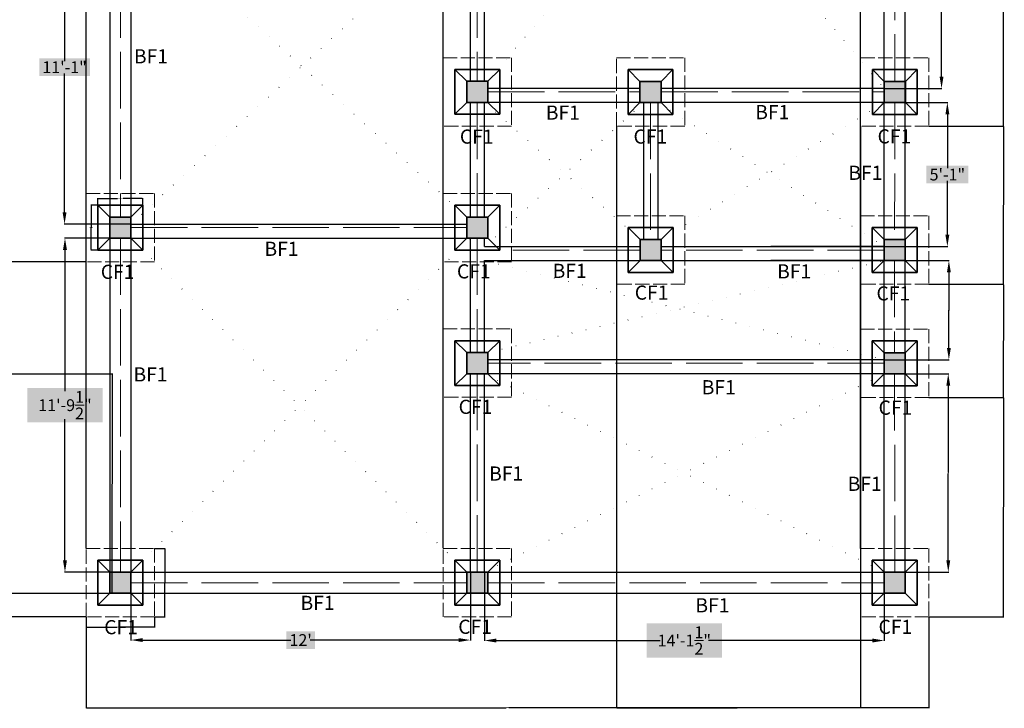
# Model space of a CAD drawing. Units: inches. Extents: x -301 to 715, y -607 to 364.
# Tile 140 of 141: x 194 to 612, y -273 to 19. Entities that reach past the tile are written whole.
import ezdxf

# ---------------------------------------------------------------- set-up
doc = ezdxf.new("R2010")
doc.units = ezdxf.units.IN
doc.header["$MEASUREMENT"] = 0
doc.linetypes.add('ACAD_ISO02W100', pattern=[15, 12, -3])
doc.linetypes.add('ACAD_ISO07W100', pattern=[3, 0, -3])
for name, color, linetype, lineweight in [('A-ANNO-DIMS', 2, 'Continuous', 18), ('S-ANNO-DIMS', 2, 'Continuous', 18), ('S-ANNO-TEXT', 240, 'Continuous', 18), ('S-BEAM-CNTR', 2, 'ACAD_ISO02W100', 13), ('S-COLS', 2, 'Continuous', 35), ('S-FNDN', 2, 'Continuous', 35), ('S-FNDN-HIDN', 220, 'ACAD_ISO02W100', 18)]:
    doc.layers.add(name, color=color, linetype=linetype, lineweight=lineweight)
for name, color, linetype, lineweight, true_color in [('S-BEAM', 152, 'Continuous', 30, 0x2776bb), ('S-COLS-PATT', 7, 'Continuous', 13, 0xffffff), ('S-FNDN-DIAG', 252, 'ACAD_ISO07W100', 13, 0x939598)]:
    doc.layers.add(name, color=color, linetype=linetype, lineweight=lineweight, true_color=true_color)
doc.styles.get("Standard").update_dxf_attribs({"font": 'arial.ttf'})
doc.dimstyles.get("Standard").update_dxf_attribs({"dimtxt": 0.18, "dimasz": 0.18, "dimexe": 0.18, "dimexo": 0.0625, "dimgap": 0.09, "dimtad": 0, "dimtih": 1, "dimtoh": 1, "dimdec": 1, "dimzin": 0, "dimdsep": 46, "dimlunit": 4, "dimtxsty": 'Standard', "dimcen": 0.09, "dimclrd": 3, "dimclre": 4, "dimclrt": 6, "dimadec": 0, "dimazin": 0, "dimtfac": 1, "dimtdec": 1, "dimtofl": 0, "dimtmove": 0, "dimatfit": 3, "dimfxl": 1, "dimtfill": 2, "dimtfillclr": 51, "dimtolj": 1, "dimtzin": 0, "dimarcsym": 0})

# ---------------------------------------------------------------- blocks, each defined once
blk = doc.blocks.new('*D58')
at = {"layer": 'Defpoints', "color": 0, "transparency": 16777216}
for p in [(391.39, -214.82), (560.9, -214.82), (560.9, -243.84)]:
    blk.add_point(p, dxfattribs=at)
at = {"layer": 'S-ANNO-DIMS', "color": 0, "lineweight": -2, "transparency": 16777216}
for p, q in [((391.39, -214.88), (391.39, -244.02)), ((560.9, -214.88), (560.9, -244.02)), ((396.39, -243.84), (465.88, -243.84)), ((555.9, -243.84), (486.41, -243.84))]:
    blk.add_line(p, q, dxfattribs=at)
at = {"layer": 'S-ANNO-DIMS', "color": 0, "transparency": 16777216}
for points in [[(396.39, -243.01), (396.39, -244.68), (391.39, -243.84)], [(555.9, -243.01), (555.9, -244.68), (560.9, -243.84)]]:
    blk.add_solid(points, dxfattribs=at)
at = {"layer": 'S-ANNO-DIMS', "color": 0, "transparency": 16777216, "insert": (476.15, -243.84), "char_height": 5, "attachment_point": 5, "bg_fill": 1, "box_fill_scale": 1.25, "bg_fill_color": 51, "bg_fill_transparency": 0}
blk.add_mtext('\\A1;14\'-1{\\H1x;\\S1/2;}"', dxfattribs=at)
blk = doc.blocks.new('*D59')
at = {"layer": 'Defpoints', "color": 0, "transparency": 16777216}
for p in [(241.39, -214.82), (385.39, -214.81), (385.39, -243.64)]:
    blk.add_point(p, dxfattribs=at)
at = {"layer": 'S-ANNO-DIMS', "color": 0, "lineweight": -2, "transparency": 16777216}
for p, q in [((241.39, -214.88), (241.39, -243.82)), ((385.39, -214.87), (385.39, -243.82)), ((246.39, -243.64), (309.29, -243.64)), ((380.39, -243.64), (317.49, -243.64))]:
    blk.add_line(p, q, dxfattribs=at)
at = {"layer": 'S-ANNO-DIMS', "color": 0, "transparency": 16777216}
for points in [[(246.39, -242.81), (246.39, -244.48), (241.39, -243.64)], [(380.39, -242.81), (380.39, -244.48), (385.39, -243.64)]]:
    blk.add_solid(points, dxfattribs=at)
at = {"layer": 'S-ANNO-DIMS', "color": 0, "transparency": 16777216, "insert": (313.39, -243.64), "char_height": 5, "attachment_point": 5, "bg_fill": 1, "box_fill_scale": 1.25, "bg_fill_color": 51, "bg_fill_transparency": 0}
blk.add_mtext("\\A1;12'", dxfattribs=at)
blk = doc.blocks.new('*D60')
at = {"layer": 'Defpoints', "color": 0, "transparency": 16777216}
for p in [(560.89, -130.82), (588.13, -130.82), (560.89, -214.82)]:
    blk.add_point(p, dxfattribs=at)
at = {"layer": 'S-ANNO-DIMS', "color": 0, "lineweight": -2, "transparency": 16777216}
for p, q in [((560.95, -130.82), (588.31, -130.82)), ((588.13, -135.82), (588.13, -172.64)), ((588.13, -209.82), (588.13, -173)), ((560.95, -214.82), (588.31, -214.82))]:
    blk.add_line(p, q, dxfattribs=at)
at = {"layer": 'S-ANNO-DIMS', "color": 0, "transparency": 16777216}
for points in [[(587.3, -135.82), (588.97, -135.82), (588.13, -130.82)], [(587.3, -209.82), (588.97, -209.82), (588.13, -214.82)]]:
    blk.add_solid(points, dxfattribs=at)
at = {"layer": 'S-ANNO-DIMS', "color": 0, "transparency": 16777216, "insert": (588.13, -172.82), "char_height": 0.18, "attachment_point": 5, "bg_fill": 1, "box_fill_scale": 1.25, "bg_fill_color": 51, "bg_fill_transparency": 0}
blk.add_mtext("\\A1;7'", dxfattribs=at)
blk = doc.blocks.new('*D61')
at = {"layer": 'Defpoints', "color": 0, "transparency": 16777216}
for p in [(560.89, -82.82), (588.39, -82.82), (560.89, -124.82)]:
    blk.add_point(p, dxfattribs=at)
at = {"layer": 'S-ANNO-DIMS', "color": 0, "lineweight": -2, "transparency": 16777216}
for p, q in [((560.95, -82.82), (588.57, -82.82)), ((588.39, -87.82), (588.39, -103.64)), ((588.39, -119.82), (588.39, -104)), ((560.95, -124.82), (588.57, -124.82))]:
    blk.add_line(p, q, dxfattribs=at)
at = {"layer": 'S-ANNO-DIMS', "color": 0, "transparency": 16777216}
for points in [[(587.56, -87.82), (589.23, -87.82), (588.39, -82.82)], [(587.56, -119.82), (589.23, -119.82), (588.39, -124.82)]]:
    blk.add_solid(points, dxfattribs=at)
at = {"layer": 'S-ANNO-DIMS', "color": 0, "transparency": 16777216, "insert": (588.39, -103.82), "char_height": 0.18, "attachment_point": 5, "bg_fill": 1, "box_fill_scale": 1.25, "bg_fill_color": 51, "bg_fill_transparency": 0}
blk.add_mtext('\\A1;3\'-6"', dxfattribs=at)
blk = doc.blocks.new('*D62')
at = {"layer": 'Defpoints', "color": 0, "transparency": 16777216}
for p in [(560.89, -15.82), (587.75, -15.82), (560.89, -76.82)]:
    blk.add_point(p, dxfattribs=at)
at = {"layer": 'S-ANNO-DIMS', "color": 0, "lineweight": -2, "transparency": 16777216}
for p, q in [((560.95, -15.82), (587.93, -15.82)), ((587.75, -20.82), (587.75, -43.67)), ((587.75, -71.82), (587.75, -48.96)), ((560.95, -76.82), (587.93, -76.82))]:
    blk.add_line(p, q, dxfattribs=at)
at = {"layer": 'S-ANNO-DIMS', "color": 0, "transparency": 16777216}
for points in [[(586.92, -20.82), (588.59, -20.82), (587.75, -15.82)], [(586.92, -71.82), (588.59, -71.82), (587.75, -76.82)]]:
    blk.add_solid(points, dxfattribs=at)
at = {"layer": 'S-ANNO-DIMS', "color": 0, "transparency": 16777216, "insert": (587.75, -46.32), "char_height": 5, "attachment_point": 5, "bg_fill": 1, "box_fill_scale": 1.25, "bg_fill_color": 51, "bg_fill_transparency": 0}
blk.add_mtext('\\A1;5\'-1"', dxfattribs=at)
blk = doc.blocks.new('*D63')
at = {"layer": 'Defpoints', "color": 0, "transparency": 16777216}
for p in [(560.89, 193.18), (585.29, 193.18), (560.89, -9.82)]:
    blk.add_point(p, dxfattribs=at)
at = {"layer": 'S-ANNO-DIMS', "color": 0, "lineweight": -2, "transparency": 16777216}
for p, q in [((560.95, 193.18), (585.47, 193.18)), ((585.29, 188.18), (585.29, 94.33)), ((585.29, -4.82), (585.29, 89.04)), ((560.95, -9.82), (585.47, -9.82))]:
    blk.add_line(p, q, dxfattribs=at)
at = {"layer": 'S-ANNO-DIMS', "color": 0, "transparency": 16777216}
for points in [[(584.46, 188.18), (586.12, 188.18), (585.29, 193.18)], [(584.46, -4.82), (586.12, -4.82), (585.29, -9.82)]]:
    blk.add_solid(points, dxfattribs=at)
at = {"layer": 'S-ANNO-DIMS', "color": 0, "transparency": 16777216, "insert": (585.29, 91.68), "char_height": 5, "attachment_point": 5, "bg_fill": 1, "box_fill_scale": 1.25, "bg_fill_color": 51, "bg_fill_transparency": 0}
blk.add_mtext('\\A1;16\'-11"', dxfattribs=at)
blk = doc.blocks.new('*D69')
at = {"layer": 'Defpoints', "color": 0, "transparency": 16777216}
for p in [(241.39, 65.68), (213.23, -67.32), (241.39, -67.32)]:
    blk.add_point(p, dxfattribs=at)
at = {"layer": 'S-ANNO-DIMS', "color": 0, "lineweight": -2, "transparency": 16777216}
for p, q in [((241.33, 65.68), (213.05, 65.68)), ((213.23, 60.68), (213.23, 1.78)), ((213.23, -62.32), (213.23, -3.42)), ((241.33, -67.32), (213.05, -67.32))]:
    blk.add_line(p, q, dxfattribs=at)
at = {"layer": 'S-ANNO-DIMS', "color": 0, "transparency": 16777216}
for points in [[(212.4, 60.68), (214.06, 60.68), (213.23, 65.68)], [(212.4, -62.32), (214.06, -62.32), (213.23, -67.32)]]:
    blk.add_solid(points, dxfattribs=at)
at = {"layer": 'S-ANNO-DIMS', "color": 0, "transparency": 16777216, "insert": (213.23, -0.82), "char_height": 5, "attachment_point": 5, "bg_fill": 1, "box_fill_scale": 1.25, "bg_fill_color": 51, "bg_fill_transparency": 0}
blk.add_mtext('\\A1;11\'-1"', dxfattribs=at)
blk = doc.blocks.new('*D70')
at = {"layer": 'Defpoints', "color": 0, "transparency": 16777216}
for p in [(241.39, -73.32), (213.4, -214.82), (241.39, -214.82)]:
    blk.add_point(p, dxfattribs=at)
at = {"layer": 'S-ANNO-DIMS', "color": 0, "lineweight": -2, "transparency": 16777216}
for p, q in [((241.33, -73.32), (213.22, -73.32)), ((213.4, -78.32), (213.4, -138.08)), ((213.4, -209.82), (213.4, -150.05)), ((241.33, -214.82), (213.22, -214.82))]:
    blk.add_line(p, q, dxfattribs=at)
at = {"layer": 'S-ANNO-DIMS', "color": 0, "transparency": 16777216}
for points in [[(212.56, -78.32), (214.23, -78.32), (213.4, -73.32)], [(212.56, -209.82), (214.23, -209.82), (213.4, -214.82)]]:
    blk.add_solid(points, dxfattribs=at)
at = {"layer": 'S-ANNO-DIMS', "color": 0, "transparency": 16777216, "insert": (213.4, -144.07), "char_height": 5, "attachment_point": 5, "bg_fill": 1, "box_fill_scale": 1.25, "bg_fill_color": 51, "bg_fill_transparency": 0}
blk.add_mtext('\\A1;11\'-9{\\H1x;\\S1/2;}"', dxfattribs=at)
blk = doc.blocks.new('CF1-BASE-29')
at = {"ltscale": 0.5}
for p, q in [((0, 0), (0, 29)), ((0, 29), (29, 29)), ((29, 29), (29, 0)), ((29, 0), (0, 0))]:
    blk.add_line(p, q, dxfattribs=at)
blk = doc.blocks.new('CF1-SLOPED-PAD')
for p, q in [((0, 0), (0, 19)), ((0, 19), (19, 19)), ((0, 19), (5, 14)), ((14, 14), (19, 19)), ((19, 19), (19, 0)), ((0, 0), (5, 5)), ((14, 5), (19, 0)), ((19, 0), (0, 0))]:
    blk.add_line(p, q)
blk = doc.blocks.new('*D92')
at = {"layer": 'A-ANNO-DIMS', "color": 4, "lineweight": -2, "transparency": 16777216}
for p, q in [((222.39, -233.88), (222.39, -238.35)), ((251.39, -233.88), (251.39, -238.35))]:
    blk.add_line(p, q, dxfattribs=at)
at = {"layer": 'A-ANNO-DIMS', "color": 3, "lineweight": -2, "transparency": 16777216}
for p, q in [((222.57, -238.17), (235.61, -238.17)), ((251.21, -238.17), (238.17, -238.17))]:
    blk.add_line(p, q, dxfattribs=at)
at = {"layer": 'A-ANNO-DIMS', "color": 3, "transparency": 16777216}
for points in [[(222.57, -238.14), (222.57, -238.2), (222.39, -238.17)], [(251.21, -238.14), (251.21, -238.2), (251.39, -238.17)]]:
    blk.add_solid(points, dxfattribs=at)
at = {"layer": 'Defpoints', "color": 0, "transparency": 16777216}
for p in [(222.39, -233.82), (251.39, -233.82), (251.39, -238.17)]:
    blk.add_point(p, dxfattribs=at)
at = {"layer": 'A-ANNO-DIMS', "color": 6, "transparency": 16777216, "insert": (236.89, -238.17), "char_height": 0.18, "attachment_point": 5, "bg_fill": 1, "box_fill_scale": 1.25, "bg_fill_color": 51, "bg_fill_transparency": 0}
blk.add_mtext('\\A1;CF1 BASE 2\'-5" TYP.', dxfattribs=at)
blk = doc.blocks.new('*D93')
at = {"layer": 'A-ANNO-DIMS', "color": 4, "lineweight": -2, "transparency": 16777216}
for p, q in [((251.45, -204.82), (255.92, -204.82)), ((251.45, -233.82), (255.92, -233.82))]:
    blk.add_line(p, q, dxfattribs=at)
at = {"layer": 'A-ANNO-DIMS', "color": 3, "lineweight": -2, "transparency": 16777216}
for p, q in [((255.74, -205), (255.74, -219.14)), ((255.74, -233.64), (255.74, -219.5))]:
    blk.add_line(p, q, dxfattribs=at)
at = {"layer": 'A-ANNO-DIMS', "color": 3, "transparency": 16777216}
for points in [[(255.71, -205), (255.77, -205), (255.74, -204.82)], [(255.71, -233.64), (255.77, -233.64), (255.74, -233.82)]]:
    blk.add_solid(points, dxfattribs=at)
at = {"layer": 'Defpoints', "color": 0, "transparency": 16777216}
for p in [(251.39, -204.82), (255.74, -204.82), (251.39, -233.82)]:
    blk.add_point(p, dxfattribs=at)
at = {"layer": 'A-ANNO-DIMS', "color": 6, "transparency": 16777216, "insert": (255.74, -219.32), "char_height": 0.18, "attachment_point": 5, "bg_fill": 1, "box_fill_scale": 1.25, "bg_fill_color": 51, "bg_fill_transparency": 0}
blk.add_mtext('\\A1;2\'-5" TYP.', dxfattribs=at)
blk = doc.blocks.new('*D94')
at = {"layer": 'A-ANNO-DIMS', "color": 4, "lineweight": -2, "transparency": 16777216}
for p, q in [((227.39, -59.26), (227.39, -56.29)), ((246.39, -59.26), (246.39, -56.29))]:
    blk.add_line(p, q, dxfattribs=at)
at = {"layer": 'A-ANNO-DIMS', "color": 3, "lineweight": -2, "transparency": 16777216}
for p, q in [((227.57, -56.47), (235.69, -56.47)), ((246.21, -56.47), (238.09, -56.47))]:
    blk.add_line(p, q, dxfattribs=at)
at = {"layer": 'A-ANNO-DIMS', "color": 3, "transparency": 16777216}
for points in [[(227.57, -56.44), (227.57, -56.5), (227.39, -56.47)], [(246.21, -56.44), (246.21, -56.5), (246.39, -56.47)]]:
    blk.add_solid(points, dxfattribs=at)
at = {"layer": 'Defpoints', "color": 0, "transparency": 16777216}
for p in [(227.39, -56.47), (227.39, -59.32), (246.39, -59.32)]:
    blk.add_point(p, dxfattribs=at)
at = {"layer": 'A-ANNO-DIMS', "color": 6, "transparency": 16777216, "insert": (236.89, -56.47), "char_height": 0.18, "attachment_point": 5, "bg_fill": 1, "box_fill_scale": 1.25, "bg_fill_color": 51, "bg_fill_transparency": 0}
blk.add_mtext('\\A1;CF1 PAD 1\'-7" TYP.', dxfattribs=at)
blk = doc.blocks.new('*D95')
at = {"layer": 'A-ANNO-DIMS', "color": 4, "lineweight": -2, "transparency": 16777216}
for p, q in [((227.33, -59.32), (224.36, -59.32)), ((227.33, -78.32), (224.36, -78.32))]:
    blk.add_line(p, q, dxfattribs=at)
at = {"layer": 'A-ANNO-DIMS', "color": 3, "lineweight": -2, "transparency": 16777216}
for p, q in [((224.54, -59.5), (224.54, -68.64)), ((224.54, -78.14), (224.54, -69))]:
    blk.add_line(p, q, dxfattribs=at)
at = {"layer": 'A-ANNO-DIMS', "color": 3, "transparency": 16777216}
for points in [[(224.51, -59.5), (224.57, -59.5), (224.54, -59.32)], [(224.51, -78.14), (224.57, -78.14), (224.54, -78.32)]]:
    blk.add_solid(points, dxfattribs=at)
at = {"layer": 'Defpoints', "color": 0, "transparency": 16777216}
for p in [(227.39, -59.32), (224.54, -78.32), (227.39, -78.32)]:
    blk.add_point(p, dxfattribs=at)
at = {"layer": 'A-ANNO-DIMS', "color": 6, "transparency": 16777216, "insert": (224.54, -68.82), "char_height": 0.18, "attachment_point": 5, "bg_fill": 1, "box_fill_scale": 1.25, "bg_fill_color": 51, "bg_fill_transparency": 0}
blk.add_mtext('\\A1;1\'-7" TYP.', dxfattribs=at)
blk = doc.blocks.new('*D152')
at = {"layer": 'A-ANNO-DIMS', "color": 4, "lineweight": -2, "transparency": 16777216}
for p, q in [((123.96, -130.82), (233.66, -130.82)), ((132.96, -223.82), (233.66, -223.82))]:
    blk.add_line(p, q, dxfattribs=at)
at = {"layer": 'A-ANNO-DIMS', "color": 3, "lineweight": -2, "transparency": 16777216}
for p, q in [((233.48, -131), (233.48, -177.14)), ((233.48, -223.64), (233.48, -177.5))]:
    blk.add_line(p, q, dxfattribs=at)
at = {"layer": 'A-ANNO-DIMS', "color": 3, "transparency": 16777216}
for points in [[(233.45, -131), (233.51, -131), (233.48, -130.82)], [(233.45, -223.64), (233.51, -223.64), (233.48, -223.82)]]:
    blk.add_solid(points, dxfattribs=at)
at = {"layer": 'Defpoints', "color": 0, "transparency": 16777216}
for p in [(123.9, -130.82), (233.48, -130.82), (132.9, -223.82)]:
    blk.add_point(p, dxfattribs=at)
at = {"layer": 'A-ANNO-DIMS', "color": 6, "transparency": 16777216, "insert": (233.48, -177.32), "char_height": 0.18, "attachment_point": 5, "bg_fill": 1, "box_fill_scale": 1.25, "bg_fill_color": 51, "bg_fill_transparency": 0}
blk.add_mtext('\\A1;7\'-9"', dxfattribs=at)
blk = doc.blocks.new('*D161')
at = {"layer": 'A-ANNO-DIMS', "color": 4, "lineweight": -2, "transparency": 16777216}
for p, q in [((222.39, -233.88), (222.39, -272.48)), ((579.9, -233.89), (579.9, -272.48))]:
    blk.add_line(p, q, dxfattribs=at)
at = {"layer": 'A-ANNO-DIMS', "color": 3, "lineweight": -2, "transparency": 16777216}
for p, q in [((222.57, -272.3), (400.54, -272.3)), ((579.72, -272.3), (401.76, -272.3))]:
    blk.add_line(p, q, dxfattribs=at)
at = {"layer": 'A-ANNO-DIMS', "color": 3, "transparency": 16777216}
for points in [[(222.57, -272.27), (222.57, -272.33), (222.39, -272.3)], [(579.72, -272.27), (579.72, -272.33), (579.9, -272.3)]]:
    blk.add_solid(points, dxfattribs=at)
at = {"layer": 'Defpoints', "color": 0, "transparency": 16777216}
for p in [(222.39, -233.82), (579.9, -233.83), (579.9, -272.3)]:
    blk.add_point(p, dxfattribs=at)
at = {"layer": 'A-ANNO-DIMS', "color": 6, "transparency": 16777216, "insert": (401.15, -272.3), "char_height": 0.18, "attachment_point": 5, "bg_fill": 1, "box_fill_scale": 1.25, "bg_fill_color": 51, "bg_fill_transparency": 0}
blk.add_mtext('\\A1;29\'-9 1/2"', dxfattribs=at)
blk = doc.blocks.new('*D162')
at = {"layer": 'A-ANNO-DIMS', "color": 4, "lineweight": -2, "transparency": 16777216}
for p, q in [((222.33, 320.18), (161.44, 320.18)), ((222.33, -233.82), (161.44, -233.82))]:
    blk.add_line(p, q, dxfattribs=at)
at = {"layer": 'A-ANNO-DIMS', "color": 3, "lineweight": -2, "transparency": 16777216}
for p, q in [((161.62, 320), (161.62, 43.36)), ((161.62, -233.64), (161.62, 43))]:
    blk.add_line(p, q, dxfattribs=at)
at = {"layer": 'A-ANNO-DIMS', "color": 3, "transparency": 16777216}
for points in [[(161.59, 320), (161.65, 320), (161.62, 320.18)], [(161.59, -233.64), (161.65, -233.64), (161.62, -233.82)]]:
    blk.add_solid(points, dxfattribs=at)
at = {"layer": 'Defpoints', "color": 0, "transparency": 16777216}
for p in [(161.62, 320.18), (222.39, 320.18), (222.39, -233.82)]:
    blk.add_point(p, dxfattribs=at)
at = {"layer": 'A-ANNO-DIMS', "color": 6, "transparency": 16777216, "insert": (161.62, 43.18), "char_height": 0.18, "attachment_point": 5, "bg_fill": 1, "box_fill_scale": 1.25, "bg_fill_color": 51, "bg_fill_transparency": 0}
blk.add_mtext('\\A1;46\'-2"', dxfattribs=at)
blk = doc.blocks.new('*D163')
at = {"layer": 'A-ANNO-DIMS', "color": 4, "lineweight": -2, "transparency": 16777216}
for p, q in [((222.39, -204.76), (222.39, 351.98)), ((373.83, -204.75), (373.83, 351.98))]:
    blk.add_line(p, q, dxfattribs=at)
at = {"layer": 'A-ANNO-DIMS', "color": 3, "lineweight": -2, "transparency": 16777216}
for p, q in [((222.57, 351.8), (297.51, 351.8)), ((373.65, 351.8), (298.71, 351.8))]:
    blk.add_line(p, q, dxfattribs=at)
at = {"layer": 'A-ANNO-DIMS', "color": 3, "transparency": 16777216}
for points in [[(222.57, 351.83), (222.57, 351.77), (222.39, 351.8)], [(373.65, 351.83), (373.65, 351.77), (373.83, 351.8)]]:
    blk.add_solid(points, dxfattribs=at)
at = {"layer": 'Defpoints', "color": 0, "transparency": 16777216}
for p in [(373.83, 351.8), (222.39, -204.82), (373.83, -204.81)]:
    blk.add_point(p, dxfattribs=at)
at = {"layer": 'A-ANNO-DIMS', "color": 6, "transparency": 16777216, "insert": (298.11, 351.8), "char_height": 0.18, "attachment_point": 5, "bg_fill": 1, "box_fill_scale": 1.25, "bg_fill_color": 51, "bg_fill_transparency": 0}
blk.add_mtext('\\A1;12\'-7 1/2"', dxfattribs=at)
blk = doc.blocks.new('*D164')
at = {"layer": 'A-ANNO-DIMS', "color": 4, "lineweight": -2, "transparency": 16777216}
for p, q in [((373.83, -204.75), (373.83, 351.98)), ((550.9, -204.77), (550.9, 351.98))]:
    blk.add_line(p, q, dxfattribs=at)
at = {"layer": 'A-ANNO-DIMS', "color": 3, "lineweight": -2, "transparency": 16777216}
for p, q in [((374.01, 351.8), (461.97, 351.8)), ((550.72, 351.8), (462.76, 351.8))]:
    blk.add_line(p, q, dxfattribs=at)
at = {"layer": 'A-ANNO-DIMS', "color": 3, "transparency": 16777216}
for points in [[(374.01, 351.83), (374.01, 351.77), (373.83, 351.8)], [(550.72, 351.83), (550.72, 351.77), (550.9, 351.8)]]:
    blk.add_solid(points, dxfattribs=at)
at = {"layer": 'Defpoints', "color": 0, "transparency": 16777216}
for p in [(550.9, 351.8), (373.83, -204.81), (550.9, -204.83)]:
    blk.add_point(p, dxfattribs=at)
at = {"layer": 'A-ANNO-DIMS', "color": 6, "transparency": 16777216, "insert": (462.36, 351.8), "char_height": 0.18, "attachment_point": 5, "bg_fill": 1, "box_fill_scale": 1.25, "bg_fill_color": 51, "bg_fill_transparency": 0}
blk.add_mtext('\\A1;14\'-9"', dxfattribs=at)
blk = doc.blocks.new('*D166')
at = {"layer": 'A-ANNO-DIMS', "color": 4, "lineweight": -2, "transparency": 16777216}
for p, q in [((447.35, -25.88), (447.35, -272.48)), ((550.92, -25.88), (550.92, -272.48))]:
    blk.add_line(p, q, dxfattribs=at)
at = {"layer": 'A-ANNO-DIMS', "color": 3, "lineweight": -2, "transparency": 16777216}
for p, q in [((447.53, -272.3), (498.6, -272.3)), ((550.74, -272.3), (499.67, -272.3))]:
    blk.add_line(p, q, dxfattribs=at)
at = {"layer": 'A-ANNO-DIMS', "color": 3, "transparency": 16777216}
for points in [[(447.53, -272.27), (447.53, -272.33), (447.35, -272.3)], [(550.74, -272.27), (550.74, -272.33), (550.92, -272.3)]]:
    blk.add_solid(points, dxfattribs=at)
at = {"layer": 'Defpoints', "color": 0, "transparency": 16777216}
for p in [(447.35, -25.82), (550.92, -25.82), (550.92, -272.3)]:
    blk.add_point(p, dxfattribs=at)
at = {"layer": 'A-ANNO-DIMS', "color": 6, "transparency": 16777216, "insert": (499.14, -272.3), "char_height": 0.18, "attachment_point": 5, "bg_fill": 1, "box_fill_scale": 1.25, "bg_fill_color": 51, "bg_fill_transparency": 0}
blk.add_mtext('\\A1;8\'-7 1/2"', dxfattribs=at)
blk = doc.blocks.new('*D167')
at = {"layer": 'A-ANNO-DIMS', "color": 4, "lineweight": -2, "transparency": 16777216}
for p, q in [((222.33, -83.32), (161.44, -83.32)), ((222.33, -233.82), (161.44, -233.82))]:
    blk.add_line(p, q, dxfattribs=at)
at = {"layer": 'A-ANNO-DIMS', "color": 3, "lineweight": -2, "transparency": 16777216}
for p, q in [((161.62, -83.5), (161.62, -158.38)), ((161.62, -233.64), (161.62, -158.75))]:
    blk.add_line(p, q, dxfattribs=at)
at = {"layer": 'A-ANNO-DIMS', "color": 3, "transparency": 16777216}
for points in [[(161.59, -83.5), (161.65, -83.5), (161.62, -83.32)], [(161.59, -233.64), (161.65, -233.64), (161.62, -233.82)]]:
    blk.add_solid(points, dxfattribs=at)
at = {"layer": 'Defpoints', "color": 0, "transparency": 16777216}
for p in [(161.62, -83.32), (222.39, -83.32), (222.39, -233.82)]:
    blk.add_point(p, dxfattribs=at)
at = {"layer": 'A-ANNO-DIMS', "color": 6, "transparency": 16777216, "insert": (161.62, -158.57), "char_height": 0.18, "attachment_point": 5, "bg_fill": 1, "box_fill_scale": 1.25, "bg_fill_color": 51, "bg_fill_transparency": 0}
blk.add_mtext('\\A1;12\'-6 1/2"', dxfattribs=at)
blk = doc.blocks.new('*D168')
at = {"layer": 'A-ANNO-DIMS', "color": 4, "lineweight": -2, "transparency": 16777216}
for p, q in [((222.33, 55.68), (161.44, 55.68)), ((222.33, -83.32), (161.44, -83.32))]:
    blk.add_line(p, q, dxfattribs=at)
at = {"layer": 'A-ANNO-DIMS', "color": 3, "lineweight": -2, "transparency": 16777216}
for p, q in [((161.62, 55.5), (161.62, -13.64)), ((161.62, -83.14), (161.62, -14))]:
    blk.add_line(p, q, dxfattribs=at)
at = {"layer": 'A-ANNO-DIMS', "color": 3, "transparency": 16777216}
for points in [[(161.59, 55.5), (161.65, 55.5), (161.62, 55.68)], [(161.59, -83.14), (161.65, -83.14), (161.62, -83.32)]]:
    blk.add_solid(points, dxfattribs=at)
at = {"layer": 'Defpoints', "color": 0, "transparency": 16777216}
for p in [(161.62, 55.68), (222.39, 55.68), (222.39, -83.32)]:
    blk.add_point(p, dxfattribs=at)
at = {"layer": 'A-ANNO-DIMS', "color": 6, "transparency": 16777216, "insert": (161.62, -13.82), "char_height": 0.18, "attachment_point": 5, "bg_fill": 1, "box_fill_scale": 1.25, "bg_fill_color": 51, "bg_fill_transparency": 0}
blk.add_mtext('\\A1;11\'-7"', dxfattribs=at)
blk = doc.blocks.new('*D171')
at = {"layer": 'A-ANNO-DIMS', "color": 4, "lineweight": -2, "transparency": 16777216}
for p, q in [((579.95, -140.82), (611.7, -140.82)), ((579.97, -233.83), (611.7, -233.83))]:
    blk.add_line(p, q, dxfattribs=at)
at = {"layer": 'A-ANNO-DIMS', "color": 3, "lineweight": -2, "transparency": 16777216}
for p, q in [((611.52, -141), (611.52, -187.14)), ((611.52, -233.65), (611.52, -187.5))]:
    blk.add_line(p, q, dxfattribs=at)
at = {"layer": 'A-ANNO-DIMS', "color": 3, "transparency": 16777216}
for points in [[(611.49, -141), (611.55, -141), (611.52, -140.82)], [(611.49, -233.65), (611.55, -233.65), (611.52, -233.83)]]:
    blk.add_solid(points, dxfattribs=at)
at = {"layer": 'Defpoints', "color": 0, "transparency": 16777216}
for p in [(579.89, -140.82), (611.52, -140.82), (579.9, -233.83)]:
    blk.add_point(p, dxfattribs=at)
at = {"layer": 'A-ANNO-DIMS', "color": 6, "transparency": 16777216, "insert": (611.52, -187.32), "char_height": 0.18, "attachment_point": 5, "bg_fill": 1, "box_fill_scale": 1.25, "bg_fill_color": 51, "bg_fill_transparency": 0}
blk.add_mtext('\\A1;7\'-9"', dxfattribs=at)
blk = doc.blocks.new('*D172')
at = {"layer": 'A-ANNO-DIMS', "color": 4, "lineweight": -2, "transparency": 16777216}
for p, q in [((579.95, -92.82), (611.7, -92.82)), ((579.95, -140.82), (611.7, -140.82))]:
    blk.add_line(p, q, dxfattribs=at)
at = {"layer": 'A-ANNO-DIMS', "color": 3, "lineweight": -2, "transparency": 16777216}
for p, q in [((611.52, -93), (611.52, -116.64)), ((611.52, -140.64), (611.52, -117))]:
    blk.add_line(p, q, dxfattribs=at)
at = {"layer": 'A-ANNO-DIMS', "color": 3, "transparency": 16777216}
for points in [[(611.49, -93), (611.55, -93), (611.52, -92.82)], [(611.49, -140.64), (611.55, -140.64), (611.52, -140.82)]]:
    blk.add_solid(points, dxfattribs=at)
at = {"layer": 'Defpoints', "color": 0, "transparency": 16777216}
for p in [(579.89, -92.82), (611.52, -92.82), (579.89, -140.82)]:
    blk.add_point(p, dxfattribs=at)
at = {"layer": 'A-ANNO-DIMS', "color": 6, "transparency": 16777216, "insert": (611.52, -116.82), "char_height": 0.18, "attachment_point": 5, "bg_fill": 1, "box_fill_scale": 1.25, "bg_fill_color": 51, "bg_fill_transparency": 0}
blk.add_mtext('\\A1;4\'-0"', dxfattribs=at)
blk = doc.blocks.new('*D173')
at = {"layer": 'A-ANNO-DIMS', "color": 4, "lineweight": -2, "transparency": 16777216}
for p, q in [((579.98, -25.82), (611.7, -25.82)), ((579.95, -92.82), (611.7, -92.82))]:
    blk.add_line(p, q, dxfattribs=at)
at = {"layer": 'A-ANNO-DIMS', "color": 3, "lineweight": -2, "transparency": 16777216}
for p, q in [((611.52, -26), (611.52, -59.14)), ((611.52, -92.64), (611.52, -59.5))]:
    blk.add_line(p, q, dxfattribs=at)
at = {"layer": 'A-ANNO-DIMS', "color": 3, "transparency": 16777216}
for points in [[(611.49, -26), (611.55, -26), (611.52, -25.82)], [(611.49, -92.64), (611.55, -92.64), (611.52, -92.82)]]:
    blk.add_solid(points, dxfattribs=at)
at = {"layer": 'Defpoints', "color": 0, "transparency": 16777216}
for p in [(579.92, -25.82), (611.52, -25.82), (579.89, -92.82)]:
    blk.add_point(p, dxfattribs=at)
at = {"layer": 'A-ANNO-DIMS', "color": 6, "transparency": 16777216, "insert": (611.52, -59.32), "char_height": 0.18, "attachment_point": 5, "bg_fill": 1, "box_fill_scale": 1.25, "bg_fill_color": 51, "bg_fill_transparency": 0}
blk.add_mtext('\\A1;5\'-7"', dxfattribs=at)
blk = doc.blocks.new('*D174')
at = {"layer": 'A-ANNO-DIMS', "color": 4, "lineweight": -2, "transparency": 16777216}
for p, q in [((579.95, 183.18), (611.7, 183.18)), ((579.98, -25.82), (611.7, -25.82))]:
    blk.add_line(p, q, dxfattribs=at)
at = {"layer": 'A-ANNO-DIMS', "color": 3, "lineweight": -2, "transparency": 16777216}
for p, q in [((611.52, 183), (611.52, 78.86)), ((611.52, -25.64), (611.52, 78.5))]:
    blk.add_line(p, q, dxfattribs=at)
at = {"layer": 'A-ANNO-DIMS', "color": 3, "transparency": 16777216}
for points in [[(611.49, 183), (611.55, 183), (611.52, 183.18)], [(611.49, -25.64), (611.55, -25.64), (611.52, -25.82)]]:
    blk.add_solid(points, dxfattribs=at)
at = {"layer": 'Defpoints', "color": 0, "transparency": 16777216}
for p in [(579.89, 183.18), (611.52, 183.18), (579.92, -25.82)]:
    blk.add_point(p, dxfattribs=at)
at = {"layer": 'A-ANNO-DIMS', "color": 6, "transparency": 16777216, "insert": (611.52, 78.68), "char_height": 0.18, "attachment_point": 5, "bg_fill": 1, "box_fill_scale": 1.25, "bg_fill_color": 51, "bg_fill_transparency": 0}
blk.add_mtext('\\A1;17\'-5"', dxfattribs=at)

msp = doc.modelspace()

# ---------------------------------------------------------------- hatches: boundary and pattern name
at = {"layer": 'S-COLS-PATT'}
h = msp.add_hatch(color=256, dxfattribs=at)
h.dxf.hatch_style = 1
h.paths.add_polyline_path([(241.39, 310.18), (232.39, 310.18), (232.39, 301.18), (241.39, 301.18)])
h.paths.add_polyline_path([(445.27, 310.18), (445.27, 301.2), (454.27, 301.2), (454.27, 310.18)])
h.paths.add_polyline_path([(560.89, 310.18), (560.89, 301.18), (569.89, 301.18), (569.89, 310.18)])
h.paths.add_polyline_path([(241.39, 202.18), (232.39, 202.18), (232.39, 193.18), (241.39, 193.18)])
h.paths.add_polyline_path([(383.81, 202.18), (383.81, 193.18), (392.81, 193.18), (392.81, 202.18)])
h.paths.add_polyline_path([(445.41, 202.18), (445.41, 193.18), (454.41, 193.18), (454.41, 202.18)])
h.paths.add_polyline_path([(560.89, 202.18), (560.89, 193.18), (569.89, 193.18), (569.89, 202.18)])
h.paths.add_polyline_path([(241.39, 65.68), (241.39, 74.68), (232.39, 74.68), (232.39, 65.68)])
h.paths.add_polyline_path([(392.83, 65.66), (392.83, 74.66), (383.83, 74.66), (383.83, 65.66)])
h.paths.add_polyline_path([(560.92, -6.82), (560.92, -15.82), (569.89, -15.82), (569.89, -9.82), (569.89, -6.82)])
h.paths.add_polyline_path([(466.35, -15.82), (466.35, -6.82), (457.35, -6.82), (457.35, -15.82)])
h.paths.add_polyline_path([(383.83, -15.78), (392.83, -15.78), (392.83, -6.78), (383.83, -6.78)])
h.paths.add_polyline_path([(241.39, -64.32), (232.39, -64.32), (232.39, -73.32), (241.39, -73.32)])
h.paths.add_polyline_path([(392.85, -64.32), (383.85, -64.32), (383.85, -73.32), (392.85, -73.32)])
h.paths.add_polyline_path([(466.37, -73.82), (457.37, -73.82), (457.37, -82.82), (466.37, -82.82)])
h.paths.add_polyline_path([(560.89, -73.82), (560.89, -82.82), (569.89, -82.82), (569.89, -73.82)])
h.paths.add_polyline_path([(560.89, -121.82), (560.89, -130.82), (569.89, -130.82), (569.89, -121.82)])
h.paths.add_polyline_path([(569.89, -214.83), (560.9, -214.83), (560.9, -223.82), (569.89, -223.82)])
h.paths.add_polyline_path([(392.83, -223.81), (392.83, -214.82), (391.39, -214.82), (385.39, -214.81), (385.39, -214.82), (383.83, -214.82), (383.83, -223.81)])
h.paths.add_polyline_path([(392.83, -121.74), (383.83, -121.74), (383.83, -130.74), (392.83, -130.74)])
h.paths.add_polyline_path([(241.39, -223.82), (241.39, -214.82), (232.39, -214.82), (232.39, -223.82)])

# ---------------------------------------------------------------- linework, layer by layer
at = {"layer": 'S-BEAM'}
for p, q in [((569.89, -9.82), (569.89, 199.18)), ((560.89, -9.82), (560.89, 193.18)), ((232.39, 71.68), (232.39, -67.32)), ((241.39, 65.68), (241.39, -67.32)), ((385.39, -6.78), (385.39, 65.66)), ((391.39, -6.82), (391.39, 65.68)), ((457.35, -9.82), (392.83, -9.82)), ((560.89, -9.82), (466.35, -9.82)), ((569.89, -76.82), (569.89, -9.82)), ((385.39, -64.32), (385.39, -15.78)), ((391.39, -64.32), (391.39, -15.82)), ((457.35, -15.82), (392.86, -15.82)), ((458.89, -15.82), (458.89, -73.82)), ((464.89, -15.82), (464.89, -73.82)), ((560.89, -15.82), (466.35, -15.82)), ((560.89, -76.82), (560.89, -15.82)), ((232.39, -67.32), (232.39, -223.82)), ((241.39, -67.32), (383.85, -67.32)), ((241.39, -73.32), (383.85, -73.32)), ((241.39, -73.32), (241.39, -214.82)), ((385.39, -121.74), (385.39, -73.32)), ((391.39, -76.82), (391.39, -73.32)), ((391.39, -76.82), (457.37, -76.82)), ((466.37, -76.82), (560.89, -76.82)), ((560.89, -76.82), (512.89, -76.82)), ((569.89, -124.82), (569.89, -76.82)), ((391.39, -121.82), (391.39, -82.82)), ((391.39, -82.82), (560.89, -82.82)), ((458.89, -82.82), (464.89, -82.82)), ((458.89, -82.82), (458.89, -82.9)), ((560.89, -82.82), (512.89, -82.82)), ((560.89, -124.82), (560.89, -82.82)), ((560.89, -124.82), (392.83, -124.82)), ((560.89, -124.82), (512.89, -124.82)), ((569.89, -223.82), (569.89, -124.82)), ((385.39, -214.82), (385.39, -130.82)), ((391.39, -214.82), (391.39, -130.82)), ((560.89, -130.82), (392.95, -130.82)), ((560.89, -214.82), (560.89, -130.82)), ((241.39, -214.82), (385.39, -214.82)), ((391.39, -214.82), (560.89, -214.82)), ((560.89, -214.82), (560.89, -214.82)), ((232.39, -223.82), (391.39, -223.82)), ((391.39, -223.82), (569.89, -223.82))]:
    msp.add_line(p, q, dxfattribs=at)
at = {"layer": 'S-BEAM-CNTR', "ltscale": 2}
for p, q in [((565.39, 193.18), (565.4, -6.82)), ((236.89, 65.68), (236.89, -64.32)), ((388.33, 65.68), (388.33, -6.78)), ((392.83, -11.28), (457.35, -11.32)), ((466.35, -11.32), (560.92, -11.32)), ((388.33, -15.78), (388.33, -64.32)), ((461.85, -15.82), (461.87, -73.82)), ((565.4, -15.82), (565.39, -73.82)), ((241.39, -68.82), (383.85, -68.82)), ((236.89, -73.32), (236.89, -214.82)), ((388.33, -73.32), (388.33, -121.74)), ((457.37, -78.34), (387.86, -78.34)), ((560.89, -78.32), (466.37, -78.34)), ((565.39, -82.82), (565.39, -121.82)), ((560.89, -126.32), (392.83, -126.24)), ((388.33, -130.74), (388.33, -214.82)), ((388.33, -130.74), (388.33, -130.82)), ((565.4, -214.83), (565.39, -130.82)), ((241.39, -219.32), (383.83, -219.32)), ((392.83, -219.32), (560.9, -219.32)), ((383.33, -223.81), (383.33, -223.82)), ((383.33, -223.81), (383.33, -223.82)), ((388.33, -223.81), (388.33, -223.82))]:
    msp.add_line(p, q, dxfattribs=at)
at = {"layer": 'S-BEAM-CNTR'}
msp.add_line((388.33, -15.78), (388.33, -15.82), dxfattribs=at)
at = {"layer": 'S-COLS'}
for p, q in [((383.83, -6.78), (392.83, -6.78)), ((383.83, -15.78), (383.83, -6.78)), ((392.83, -6.78), (392.83, -15.78)), ((457.35, -6.82), (466.35, -6.82)), ((457.35, -15.82), (457.35, -6.82)), ((466.35, -6.82), (466.35, -15.82)), ((560.92, -6.82), (569.92, -6.82)), ((560.92, -15.82), (560.92, -6.82)), ((569.92, -6.82), (569.92, -15.82)), ((392.83, -15.78), (383.83, -15.78)), ((466.35, -15.82), (457.35, -15.82)), ((569.92, -15.82), (560.92, -15.82)), ((232.39, -64.32), (241.39, -64.32)), ((232.39, -73.32), (232.39, -64.32)), ((241.39, -64.32), (241.39, -73.32)), ((383.85, -64.32), (392.85, -64.32)), ((383.85, -73.32), (383.85, -64.32)), ((392.85, -64.32), (392.85, -73.32)), ((241.39, -73.32), (232.39, -73.32)), ((392.85, -73.32), (383.85, -73.32)), ((457.37, -73.82), (466.37, -73.82)), ((457.37, -82.82), (457.37, -73.82)), ((466.37, -73.82), (466.37, -82.82)), ((560.89, -73.82), (569.89, -73.82)), ((560.89, -82.82), (560.89, -73.82)), ((569.89, -73.82), (569.89, -82.82)), ((466.37, -82.82), (457.37, -82.82)), ((569.89, -82.82), (560.89, -82.82)), ((383.83, -121.74), (392.83, -121.74)), ((383.83, -130.74), (383.83, -121.74)), ((392.83, -121.74), (392.83, -130.74)), ((560.89, -121.82), (569.89, -121.82)), ((560.89, -130.82), (560.89, -121.82)), ((569.89, -121.82), (569.89, -130.82)), ((392.83, -130.74), (383.83, -130.74)), ((569.89, -130.82), (560.89, -130.82)), ((232.39, -214.82), (241.39, -214.82)), ((232.39, -223.82), (232.39, -214.82)), ((241.39, -214.82), (241.39, -223.82)), ((383.83, -214.81), (392.83, -214.81)), ((383.83, -223.81), (383.83, -214.81)), ((392.83, -214.81), (392.83, -223.81)), ((560.9, -214.83), (569.9, -214.83)), ((560.9, -223.83), (560.9, -214.83)), ((569.9, -214.83), (569.9, -223.83)), ((241.39, -223.82), (232.39, -223.82)), ((392.83, -223.81), (383.83, -223.81)), ((569.9, -223.83), (560.9, -223.83))]:
    msp.add_line(p, q, dxfattribs=at)
at = {"layer": 'S-FNDN'}
for p, q in [((555.92, -20.82), (555.92, -1.82)), ((555.92, -1.82), (574.92, -1.82)), ((555.92, -1.82), (560.92, -6.82)), ((569.92, -6.82), (574.92, -1.82)), ((574.92, -1.82), (574.92, -20.82)), ((555.92, -20.82), (560.89, -15.82)), ((569.92, -15.82), (574.92, -20.82)), ((574.92, -20.82), (555.92, -20.82)), ((555.9, -228.83), (555.9, -209.83)), ((555.9, -209.83), (574.9, -209.83)), ((560.89, -214.82), (555.9, -209.83)), ((569.9, -214.83), (574.9, -209.83)), ((574.9, -209.83), (574.9, -228.83)), ((555.9, -228.83), (560.9, -223.83)), ((569.89, -223.82), (574.9, -228.83)), ((574.9, -228.83), (555.9, -228.83))]:
    msp.add_line(p, q, dxfattribs=at)
at = {"layer": 'S-FNDN-DIAG', "ltscale": 2}
for p, q in [((391.39, 193.18), (560.89, -9.82)), ((392.83, -6.78), (560.89, 193.18)), ((241.39, 65.68), (383.85, -64.32)), ((241.39, -67.32), (385.39, 65.66)), ((391.39, -76.82), (458.89, -15.82)), ((391.39, -15.82), (457.37, -73.82)), ((464.89, -15.82), (560.89, -76.82)), ((466.37, -73.82), (560.89, -15.82)), ((241.39, -214.82), (385.39, -73.32)), ((241.39, -73.32), (383.83, -214.82)), ((391.39, -82.82), (560.89, -124.82)), ((392.83, -121.74), (560.89, -82.82)), ((391.39, -214.82), (560.89, -130.82)), ((391.39, -130.82), (560.89, -214.82))]:
    msp.add_line(p, q, dxfattribs=at)

# ---------------------------------------------------------------- block references
at = {"layer": 'S-FNDN'}
for p, rotation in [((397.83, -1.78), 180), ((452.35, -1.82), 269.9999999999995), ((246.39, -59.32), 180), ((397.85, -59.32), 180), ((471.37, -68.82), 180), ((555.89, -68.82), 269.9999999999998), ((397.83, -116.74), 180), ((378.83, -209.81), 270.0000000000001)]:
    msp.add_blockref('CF1-SLOPED-PAD', p, dxfattribs=dict(at, rotation=rotation))
for p in [(555.89, -135.82), (227.39, -228.82)]:
    msp.add_blockref('CF1-SLOPED-PAD', p, dxfattribs=at)
at = {"layer": 'S-FNDN-HIDN'}
for p in [(373.83, -25.78), (550.92, -25.82), (222.39, -83.32), (373.85, -83.32), (447.37, -92.82), (373.83, -140.74), (222.39, -233.82), (550.9, -233.83)]:
    msp.add_blockref('CF1-BASE-29', p, dxfattribs=at)
for p, rotation in [((476.35, -25.82), 90.00000000000011), ((579.89, -92.82), 89.99999999999974), ((579.89, -111.82), 180), ((402.83, -233.81), 90.00000000000018)]:
    msp.add_blockref('CF1-BASE-29', p, dxfattribs=dict(at, rotation=rotation))

# ---------------------------------------------------------------- texts
at = {"layer": 'S-ANNO-TEXT'}
for s, p in [('BF1', (242.64, 0.82)), ('BF1', (417.4, -23.05)), ('BF1', (506.24, -22.84)), ('CF1', (380.92, -33.22)), ('CF1', (454.59, -33.21)), ('CF1', (558.14, -33.15)), ('BF1', (545.76, -48.58)), ('BF1', (298.03, -80.79)), ('CF1', (228.58, -90.55)), ('CF1', (379.69, -90.36)), ('BF1', (420.29, -90.14)), ('BF1', (515.53, -90.36)), ('CF1', (455.13, -99.36)), ('CF1', (557.67, -99.7)), ('BF1', (242.46, -134.04)), ('BF1', (483.54, -139.47)), ('CF1', (380.4, -147.78)), ('CF1', (558.57, -148.13)), ('BF1', (393.34, -176.06)), ('BF1', (545.47, -180.41)), ('BF1', (313.33, -230.88)), ('BF1', (480.86, -231.9)), ('CF1', (230.06, -241.18)), ('CF1', (380.25, -241.01)), ('CF1', (558.55, -241.05))]:
    msp.add_text(s, height=6, dxfattribs=at).set_placement(p)

# ---------------------------------------------------------------- dimensions: what is measured, and where the dimension line sits
at = {"layer": 'A-ANNO-DIMS'}
for base, p1, p2, picture, middle in [((373.83, 351.8), (222.39, -204.82), (373.83, -204.81), '*D163', (298.11, 351.8)), ((550.9, 351.8), (373.83, -204.81), (550.9, -204.83), '*D164', (462.36, 351.8)), ((550.92, -272.3), (447.35, -25.82), (550.92, -25.82), '*D166', (499.14, -272.3)), ((579.9, -272.3), (222.39, -233.82), (579.9, -233.83), '*D161', (401.15, -272.3))]:
    dim = msp.add_linear_dim(base=base, p1=p1, p2=p2, dimstyle='Standard', override={"dimdec": 1, "dimlfac": 1, "dimrnd": 0, "dimzin": 1, "dimdsep": 46, "dimlunit": 4, "dimfrac": 2}, dxfattribs=at)
    dim.commit()
    dim.dimension.update_dxf_attribs({"geometry": picture, "text_midpoint": middle})
for base, p1, p2, picture, middle in [((161.62, 320.18), (222.39, -233.82), (222.39, 320.18), '*D162', (161.62, 43.18)), ((611.52, 183.18), (579.92, -25.82), (579.89, 183.18), '*D174', (611.52, 78.68)), ((161.62, 55.68), (222.39, -83.32), (222.39, 55.68), '*D168', (161.62, -13.82)), ((611.52, -25.82), (579.89, -92.82), (579.92, -25.82), '*D173', (611.52, -59.32)), ((161.62, -83.32), (222.39, -233.82), (222.39, -83.32), '*D167', (161.62, -158.57)), ((611.52, -92.82), (579.89, -140.82), (579.89, -92.82), '*D172', (611.52, -116.82)), ((233.48, -130.82), (132.9, -223.82), (123.9, -130.82), '*D152', (233.48, -177.32)), ((611.52, -140.82), (579.9, -233.83), (579.89, -140.82), '*D171', (611.52, -187.32))]:
    dim = msp.add_linear_dim(base=base, p1=p1, p2=p2, angle=90, dimstyle='Standard', override={"dimdec": 1, "dimlfac": 1, "dimrnd": 0, "dimzin": 1, "dimdsep": 46, "dimlunit": 4, "dimfrac": 2}, dxfattribs=at)
    dim.commit()
    dim.dimension.update_dxf_attribs({"geometry": picture, "text_midpoint": middle})
for base, p1, p2, angle, text, picture, middle in [((227.39, -56.47), (246.39, -59.32), (227.39, -59.32), 180, 'CF1 PAD <> TYP.', '*D94', (236.89, -56.47)), ((224.54, -78.32), (227.39, -59.32), (227.39, -78.32), 270, '<> TYP.', '*D95', (224.54, -68.82)), ((255.74, -204.82), (251.39, -233.82), (251.39, -204.82), 90, '<> TYP.', '*D93', (255.74, -219.32))]:
    dim = msp.add_linear_dim(base=base, p1=p1, p2=p2, angle=angle, text=text, dimstyle='Standard', override={"dimdec": 1, "dimlfac": 1, "dimrnd": 0, "dimzin": 1, "dimdsep": 46, "dimlunit": 4, "dimfrac": 2}, dxfattribs=at)
    dim.commit()
    dim.dimension.update_dxf_attribs({"geometry": picture, "text_midpoint": middle})
dim = msp.add_linear_dim(base=(251.39, -238.17), p1=(222.39, -233.82), p2=(251.39, -233.82), text='CF1 BASE <> TYP.', dimstyle='Standard', override={"dimdec": 1, "dimlfac": 1, "dimrnd": 0, "dimzin": 1, "dimdsep": 46, "dimlunit": 4, "dimfrac": 2}, dxfattribs=at)
dim.commit()
dim.dimension.update_dxf_attribs({"geometry": '*D92', "text_midpoint": (236.89, -238.17)})
at = {"layer": 'S-ANNO-DIMS'}
for base, p1, p2, override, picture, middle in [((585.29, 193.18), (560.89, -9.82), (560.89, 193.18), {"dimtxt": 5, "dimasz": 5, "dimclrd": 0, "dimclre": 0, "dimclrt": 0}, '*D63', (585.29, 91.68)), ((213.23, -67.32), (241.39, 65.68), (241.39, -67.32), {"dimtxt": 5, "dimasz": 5, "dimclrd": 0, "dimclre": 0, "dimclrt": 0}, '*D69', (213.23, -0.82)), ((587.75, -15.82), (560.89, -76.82), (560.89, -15.82), {"dimtxt": 5, "dimasz": 5, "dimclrd": 0, "dimclre": 0, "dimclrt": 0}, '*D62', (587.75, -46.32)), ((213.4, -214.82), (241.39, -73.32), (241.39, -214.82), {"dimtxt": 5, "dimasz": 5, "dimclrd": 0, "dimclre": 0, "dimclrt": 0}, '*D70', (213.4, -144.07)), ((588.39, -82.82), (560.89, -124.82), (560.89, -82.82), {"dimasz": 5, "dimclrd": 0, "dimclre": 0, "dimclrt": 0}, '*D61', (588.39, -103.82)), ((588.13, -130.82), (560.89, -214.82), (560.89, -130.82), {"dimasz": 5, "dimclrd": 0, "dimclre": 0, "dimclrt": 0}, '*D60', (588.13, -172.82))]:
    dim = msp.add_linear_dim(base=base, p1=p1, p2=p2, angle=90, dimstyle='Standard', override=override, dxfattribs=at)
    dim.commit()
    dim.dimension.update_dxf_attribs({"geometry": picture, "text_midpoint": middle})
for base, p1, p2, picture, middle in [((385.39, -243.64), (241.39, -214.82), (385.39, -214.81), '*D59', (313.39, -243.64)), ((560.9, -243.84), (391.39, -214.82), (560.9, -214.82), '*D58', (476.15, -243.84))]:
    dim = msp.add_linear_dim(base=base, p1=p1, p2=p2, dimstyle='Standard', override={"dimtxt": 5, "dimasz": 5, "dimclrd": 0, "dimclre": 0, "dimclrt": 0}, dxfattribs=at)
    dim.commit()
    dim.dimension.update_dxf_attribs({"geometry": picture, "text_midpoint": middle})

doc.saveas('drawing.dxf')
